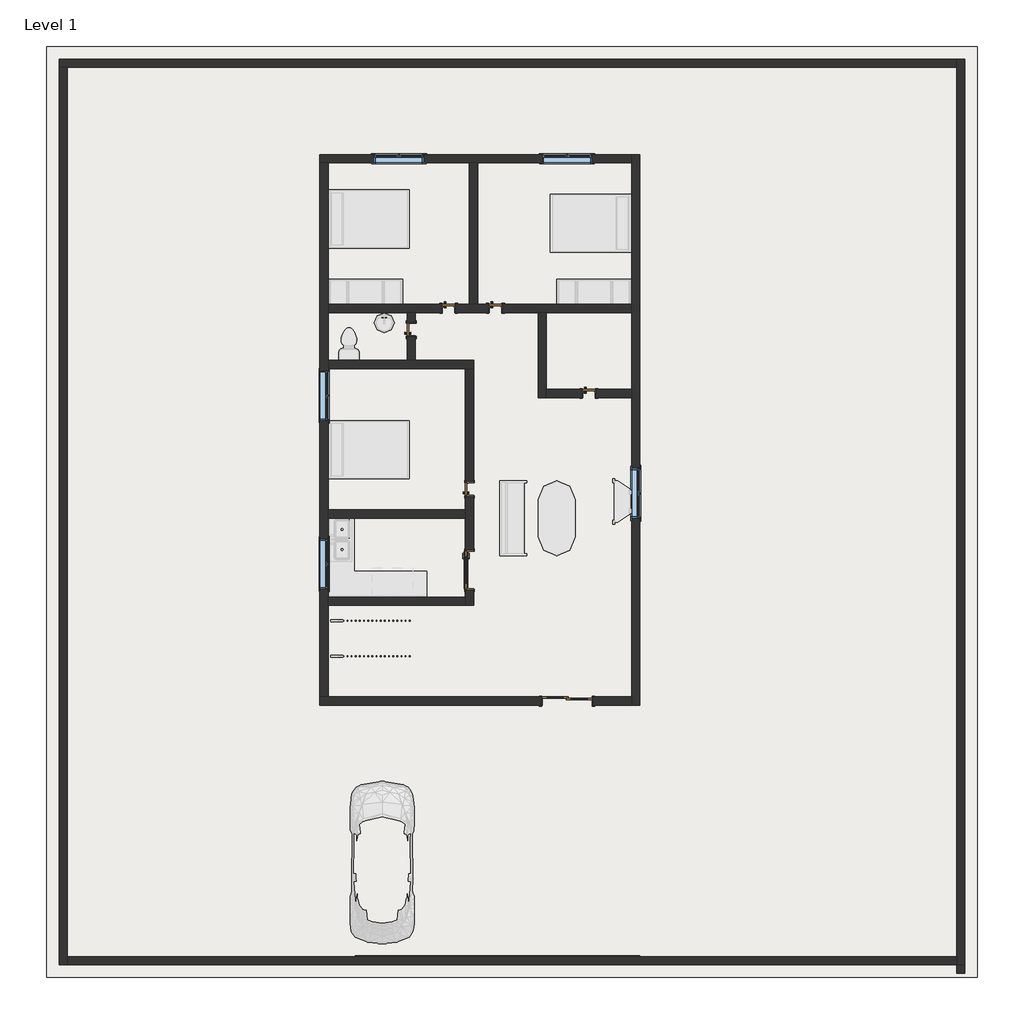
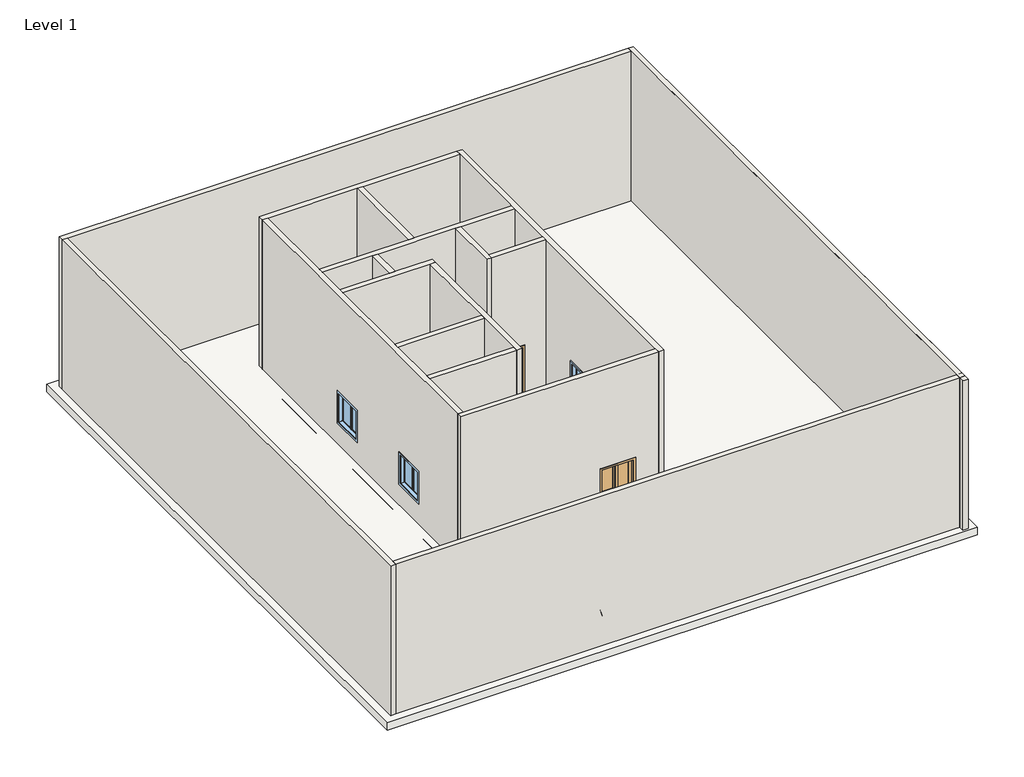
# One storey, part 1 of 3: 21 walls, 7 doors, 5 windows, 2 slabs.
"""IFC4 building model written with IfcOpenShell, lengths in millimetres."""

from ifc_helpers import new_model, si_unit, frame, origin, origin_with_axes, place, context, project, spatial, polyline, outline, extrude, faceted_brep, transform, mapped, element, save
from components import door_1768e003, door_f9cb40a9, door_5a382651, window_0862ab64

model = new_model("IFC4")

# Units and contexts
model_context = context("Model", 3, world=origin())
ifc_project = project(units=[si_unit("LENGTHUNIT", "METRE", prefix="MILLI")], contexts=[model_context])

# Site, building, storey
site = spatial("IfcSite", under=ifc_project)
building = spatial("IfcBuilding", under=site)
storey = spatial("IfcBuildingStorey", under=building, Name="Level 1", Elevation=0.0)

# Doors
placement = place(None, origin())
door_shape = door_1768e003(model_context)
element("IfcDoor", 1, ObjectType="36\" x 80\"", at=placement, inside=storey, context=model_context, shape_type="MappedRepresentation", body=[
    mapped(door_shape, transform((-7446.4010462, -2064.5818688, 0.0), x_axis=(0.0, 1.0, 0.0), y_axis=(-1.0, 0.0, 0.0), z_axis=(0.0, 0.0, 1.0))),
])
door_2_shape = door_f9cb40a9(model_context)
element("IfcDoor", 2, ObjectType="Door-Interior-Double-Sliding-2_Panel-Wood : 48\" x 80\"", at=placement, inside=storey, context=model_context, shape_type="MappedRepresentation", body=[
    mapped(door_2_shape, transform((-5055.6260462, -5261.8068688, 0.0), x_axis=(1.0, 0.0, 0.0), y_axis=(0.0, 1.0, 0.0), z_axis=(0.0, 0.0, 1.0))),
])
door_3_shape = door_5a382651(model_context)
element("IfcDoor", 3, ObjectType="Door-Interior-Single-5_Panel_Vert-Wood : 12\" x 80\"", at=placement, inside=storey, context=model_context, shape_type="MappedRepresentation", body=[
    mapped(door_3_shape, transform((-7951.2260462, 4339.3931312, 0.0), x_axis=(1.0, 0.0, 0.0), y_axis=(0.0, 1.0, 0.0), z_axis=(0.0, 0.0, 1.0))),
])
element("IfcDoor", 4, ObjectType="Door-Interior-Single-5_Panel_Vert-Wood : 12\" x 80\"", at=placement, inside=storey, context=model_context, shape_type="MappedRepresentation", body=[
    mapped(door_3_shape, transform((-6808.2260462, 4339.3931312, 0.0), x_axis=(1.0, 0.0, 0.0), y_axis=(0.0, 1.0, 0.0), z_axis=(0.0, 0.0, 1.0))),
])
element("IfcDoor", 5, ObjectType="Door-Interior-Single-5_Panel_Vert-Wood : 12\" x 80\"", at=placement, inside=storey, context=model_context, shape_type="MappedRepresentation", body=[
    mapped(door_3_shape, transform((-8868.8010462, 3815.5181312, 0.0), x_axis=(0.0, 1.0, 0.0), y_axis=(-1.0, 0.0, 0.0), z_axis=(0.0, 0.0, 1.0))),
])
element("IfcDoor", 6, ObjectType="Door-Interior-Single-5_Panel_Vert-Wood : 12\" x 80\"", at=placement, inside=storey, context=model_context, shape_type="MappedRepresentation", body=[
    mapped(door_3_shape, transform((-4522.2260462, 2256.5931312, 0.0), x_axis=(1.0, 0.0, 0.0), y_axis=(0.0, 1.0, 0.0), z_axis=(0.0, 0.0, 1.0))),
])
element("IfcDoor", 7, ObjectType="Door-Interior-Single-5_Panel_Vert-Wood : 12\" x 80\"", at=placement, inside=storey, context=model_context, shape_type="MappedRepresentation", body=[
    mapped(door_3_shape, transform((-7446.4010462, -83.3818688, 0.0), x_axis=(0.0, 1.0, 0.0), y_axis=(-1.0, 0.0, 0.0), z_axis=(0.0, 0.0, 1.0))),
])

# Slabs
element("IfcSlab", 8, ObjectType="Generic - 12\"", at=placement, inside=storey, context=model_context, shape_type="SweptSolid", body=[
    extrude(outline(polyline([(-11405.6260462, 8400.2181312), (-2972.8260462, 8400.2181312), (-2972.8260462, -5671.3818688), (-11405.6260462, -5671.3818688), (-11405.6260462, 8400.2181312)])), frame((0.0, 0.0, -304.8), z_axis=(0.0, 0.0, 1.0), x_axis=(1.0, 0.0, 0.0)), (0.0, 0.0, 1.0), 304.8),
])
element("IfcSlab", 9, ObjectType="Generic - 12\"", at=placement, inside=storey, context=model_context, shape_type="SweptSolid", body=[
    extrude(outline(polyline([(-17782.399436, -12021.3818688), (-17782.399436, 10737.0181312), (4976.000564, 10737.0181312), (4976.000564, -12021.3818688), (-17782.399436, -12021.3818688)])), frame((0.0, 0.0, -304.8), z_axis=(0.0, 0.0, 1.0), x_axis=(1.0, 0.0, 0.0)), (0.0, 0.0, 1.0), 304.8),
])

# Walls
element("IfcWall", 10, ObjectType="Generic - 8\"", at=placement, inside=storey, context=model_context, shape_type="Brep", body=[
    faceted_brep([(-11100.8260462, 7892.2181312, 0.0), (-10897.6260462, 7892.2181312, 0.0), (-7443.2260462, 7892.2181312, 0.0), (-7240.0260462, 7892.2181312, 0.0), (-3480.8260462, 7892.2181312, 0.0), (-3480.8260462, 7892.2181312, 6096.0), (-7240.0260462, 7892.2181312, 6096.0), (-7443.2260462, 7892.2181312, 6096.0), (-10897.6260462, 7892.2181312, 6096.0), (-11100.8260462, 7892.2181312, 6096.0), (-8560.8260462, 7892.2181312, 2133.6), (-8560.8260462, 7892.2181312, 914.4), (-9780.0260462, 7892.2181312, 914.4), (-9780.0260462, 7892.2181312, 2133.6), (-4446.0260462, 7892.2181312, 2133.6), (-4446.0260462, 7892.2181312, 914.4), (-5665.2260462, 7892.2181312, 914.4), (-5665.2260462, 7892.2181312, 2133.6), (-11100.8260462, 8095.4181312, 0.0), (-11100.8260462, 8095.4181312, 6096.0), (-3480.8260462, 8095.4181312, 6096.0), (-3480.8260462, 8095.4181312, 0.0), (-8560.8260462, 8095.4181312, 2133.6), (-9780.0260462, 8095.4181312, 2133.6), (-9780.0260462, 8095.4181312, 914.4), (-8560.8260462, 8095.4181312, 914.4), (-4446.0260462, 8095.4181312, 2133.6), (-5665.2260462, 8095.4181312, 2133.6), (-5665.2260462, 8095.4181312, 914.4), (-4446.0260462, 8095.4181312, 914.4)], [[[0, 1, 2, 3, 4, 5, 6, 7, 8, 9], [10, 11, 12, 13], [14, 15, 16, 17]], [[18, 19, 20, 21], [22, 23, 24, 25], [26, 27, 28, 29]], [[4, 3, 2, 1, 0, 18, 21]], [[9, 8, 7, 6, 5, 20, 19]], [[0, 9, 19, 18]], [[5, 4, 21, 20]], [[11, 10, 22, 25]], [[12, 11, 25, 24]], [[13, 12, 24, 23]], [[10, 13, 23, 22]], [[15, 14, 26, 29]], [[16, 15, 29, 28]], [[17, 16, 28, 27]], [[14, 17, 27, 26]]]),
])
element("IfcWall", 11, ObjectType="Generic - 8\"", at=placement, inside=storey, context=model_context, shape_type="Brep", body=[
    faceted_brep([(-3480.8260462, 8095.4181312, 0.0), (-3480.8260462, 7892.2181312, 0.0), (-3480.8260462, 4437.8181312, 0.0), (-3480.8260462, 4234.6181312, 0.0), (-3480.8260462, 2355.0181312, 0.0), (-3480.8260462, 2151.8181312, 0.0), (-3480.8260462, -5163.3818688, 0.0), (-3480.8260462, -5366.5818688, 0.0), (-3480.8260462, -5366.5818688, 6096.0), (-3480.8260462, -5163.3818688, 6096.0), (-3480.8260462, 2151.8181312, 6096.0), (-3480.8260462, 2355.0181312, 6096.0), (-3480.8260462, 4234.6181312, 6096.0), (-3480.8260462, 4437.8181312, 6096.0), (-3480.8260462, 7892.2181312, 6096.0), (-3480.8260462, 8095.4181312, 6096.0), (-3480.8260462, -794.5818688, 2133.6), (-3480.8260462, -794.5818688, 914.4), (-3480.8260462, 424.6181312, 914.4), (-3480.8260462, 424.6181312, 2133.6), (-3277.6260462, 8095.4181312, 0.0), (-3277.6260462, 8095.4181312, 6096.0), (-3277.6260462, -5366.5818688, 6096.0), (-3277.6260462, -5366.5818688, 0.0), (-3277.6260462, -794.5818688, 2133.6), (-3277.6260462, 424.6181312, 2133.6), (-3277.6260462, 424.6181312, 914.4), (-3277.6260462, -794.5818688, 914.4)], [[[0, 1, 2, 3, 4, 5, 6, 7, 8, 9, 10, 11, 12, 13, 14, 15], [16, 17, 18, 19]], [[20, 21, 22, 23], [24, 25, 26, 27]], [[7, 6, 5, 4, 3, 2, 1, 0, 20, 23]], [[15, 14, 13, 12, 11, 10, 9, 8, 22, 21]], [[8, 7, 23, 22]], [[0, 15, 21, 20]], [[17, 16, 24, 27]], [[18, 17, 27, 26]], [[19, 18, 26, 25]], [[16, 19, 25, 24]]]),
])
element("IfcWall", 12, ObjectType="Generic - 8\"", at=placement, inside=storey, context=model_context, shape_type="Brep", body=[
    faceted_brep([(-11100.8260462, -5163.3818688, 6096.0), (-10897.6260462, -5163.3818688, 6096.0), (-3480.8260462, -5163.3818688, 6096.0), (-3480.8260462, -5163.3818688, 0.0), (-4420.6260462, -5163.3818688, 0.0), (-4420.6260462, -5163.3818688, 2057.4), (-5690.6260462, -5163.3818688, 2057.4), (-5690.6260462, -5163.3818688, 0.0), (-10897.6260462, -5163.3818688, 0.0), (-11100.8260462, -5163.3818688, 0.0), (-3480.8260462, -5366.5818688, 6096.0), (-11100.8260462, -5366.5818688, 6096.0), (-11100.8260462, -5366.5818688, 0.0), (-5690.6260462, -5366.5818688, 0.0), (-5690.6260462, -5366.5818688, 2057.4), (-4420.6260462, -5366.5818688, 2057.4), (-4420.6260462, -5366.5818688, 0.0), (-3480.8260462, -5366.5818688, 0.0)], [[[0, 1, 2, 3, 4, 5, 6, 7, 8, 9]], [[10, 11, 12, 13, 14, 15, 16, 17]], [[3, 17, 16, 4]], [[12, 9, 8, 7, 13]], [[2, 1, 0, 11, 10]], [[3, 2, 10, 17]], [[0, 9, 12, 11]], [[15, 5, 4, 16]], [[5, 15, 14, 6]], [[6, 14, 13, 7]]]),
])
element("IfcWall", 13, ObjectType="Generic - 8\"", at=placement, inside=storey, context=model_context, shape_type="Brep", body=[
    faceted_brep([(-10897.6260462, -5163.3818688, 0.0), (-10897.6260462, -2928.1818688, 0.0), (-10897.6260462, -2724.9818688, 0.0), (-10897.6260462, -794.5818688, 0.0), (-10897.6260462, -591.3818688, 0.0), (-10897.6260462, 2863.0181312, 0.0), (-10897.6260462, 3066.2181312, 0.0), (-10897.6260462, 4234.6181312, 0.0), (-10897.6260462, 4437.8181312, 0.0), (-10897.6260462, 7892.2181312, 0.0), (-10897.6260462, 7892.2181312, 6096.0), (-10897.6260462, 4437.8181312, 6096.0), (-10897.6260462, 4234.6181312, 6096.0), (-10897.6260462, 3066.2181312, 6096.0), (-10897.6260462, 2863.0181312, 6096.0), (-10897.6260462, -591.3818688, 6096.0), (-10897.6260462, -794.5818688, 6096.0), (-10897.6260462, -2724.9818688, 6096.0), (-10897.6260462, -2928.1818688, 6096.0), (-10897.6260462, -5163.3818688, 6096.0), (-10897.6260462, -2521.7818688, 2133.6), (-10897.6260462, -1302.5818688, 2133.6), (-10897.6260462, -1302.5818688, 914.4), (-10897.6260462, -2521.7818688, 914.4), (-10897.6260462, 1593.0181312, 2133.6), (-10897.6260462, 2812.2181312, 2133.6), (-10897.6260462, 2812.2181312, 914.4), (-10897.6260462, 1593.0181312, 914.4), (-11100.8260462, -5163.3818688, 0.0), (-11100.8260462, -5163.3818688, 6096.0), (-11100.8260462, 7892.2181312, 6096.0), (-11100.8260462, 7892.2181312, 0.0), (-11100.8260462, -2521.7818688, 2133.6), (-11100.8260462, -2521.7818688, 914.4), (-11100.8260462, -1302.5818688, 914.4), (-11100.8260462, -1302.5818688, 2133.6), (-11100.8260462, 1593.0181312, 2133.6), (-11100.8260462, 1593.0181312, 914.4), (-11100.8260462, 2812.2181312, 914.4), (-11100.8260462, 2812.2181312, 2133.6)], [[[0, 1, 2, 3, 4, 5, 6, 7, 8, 9, 10, 11, 12, 13, 14, 15, 16, 17, 18, 19], [20, 21, 22, 23], [24, 25, 26, 27]], [[28, 29, 30, 31], [32, 33, 34, 35], [36, 37, 38, 39]], [[9, 8, 7, 6, 5, 4, 3, 2, 1, 0, 28, 31]], [[19, 18, 17, 16, 15, 14, 13, 12, 11, 10, 30, 29]], [[10, 9, 31, 30]], [[0, 19, 29, 28]], [[33, 32, 20, 23]], [[34, 33, 23, 22]], [[35, 34, 22, 21]], [[32, 35, 21, 20]], [[37, 36, 24, 27]], [[38, 37, 27, 26]], [[39, 38, 26, 25]], [[36, 39, 25, 24]]]),
])
element("IfcWall", 14, ObjectType="Generic - 8\"", at=placement, inside=storey, context=model_context, shape_type="Brep", body=[
    faceted_brep([(-3480.8260462, 4234.6181312, 6096.0), (-5563.6260462, 4234.6181312, 6096.0), (-5766.8260462, 4234.6181312, 6096.0), (-8764.0260462, 4234.6181312, 6096.0), (-8967.2260462, 4234.6181312, 6096.0), (-10897.6260462, 4234.6181312, 6096.0), (-10897.6260462, 4234.6181312, 0.0), (-8967.2260462, 4234.6181312, 0.0), (-8764.0260462, 4234.6181312, 0.0), (-8129.0260462, 4234.6181312, 0.0), (-8129.0260462, 4234.6181312, 2057.4), (-7773.4260462, 4234.6181312, 2057.4), (-7773.4260462, 4234.6181312, 0.0), (-6986.0260462, 4234.6181312, 0.0), (-6986.0260462, 4234.6181312, 2057.4), (-6630.4260462, 4234.6181312, 2057.4), (-6630.4260462, 4234.6181312, 0.0), (-5766.8260462, 4234.6181312, 0.0), (-5563.6260462, 4234.6181312, 0.0), (-3480.8260462, 4234.6181312, 0.0), (-10897.6260462, 4437.8181312, 6096.0), (-7443.2260462, 4437.8181312, 6096.0), (-7240.0260462, 4437.8181312, 6096.0), (-3480.8260462, 4437.8181312, 6096.0), (-3480.8260462, 4437.8181312, 0.0), (-6630.4260462, 4437.8181312, 0.0), (-6630.4260462, 4437.8181312, 2057.4), (-6986.0260462, 4437.8181312, 2057.4), (-6986.0260462, 4437.8181312, 0.0), (-7240.0260462, 4437.8181312, 0.0), (-7443.2260462, 4437.8181312, 0.0), (-7773.4260462, 4437.8181312, 0.0), (-7773.4260462, 4437.8181312, 2057.4), (-8129.0260462, 4437.8181312, 2057.4), (-8129.0260462, 4437.8181312, 0.0), (-10897.6260462, 4437.8181312, 0.0)], [[[0, 1, 2, 3, 4, 5, 6, 7, 8, 9, 10, 11, 12, 13, 14, 15, 16, 17, 18, 19]], [[20, 21, 22, 23, 24, 25, 26, 27, 28, 29, 30, 31, 32, 33, 34, 35]], [[6, 35, 34, 9, 8, 7]], [[24, 19, 18, 17, 16, 25]], [[12, 31, 30, 29, 28, 13]], [[5, 4, 3, 2, 1, 0, 23, 22, 21, 20]], [[0, 19, 24, 23]], [[6, 5, 20, 35]], [[11, 32, 31, 12]], [[32, 11, 10, 33]], [[33, 10, 9, 34]], [[15, 26, 25, 16]], [[26, 15, 14, 27]], [[27, 14, 13, 28]]]),
])
element("IfcWall", 15, ObjectType="Generic - 8\"", at=placement, inside=storey, context=model_context, shape_type="SweptSolid", body=[
    extrude(outline(polyline([(-7443.2260462, 7892.2181312), (-7240.0260462, 7892.2181312), (-7240.0260462, 4437.8181312), (-7443.2260462, 4437.8181312), (-7443.2260462, 7892.2181312)])), origin_with_axes(), (0.0, 0.0, 1.0), 6096.0),
])
element("IfcWall", 16, ObjectType="Generic - 8\"", at=placement, inside=storey, context=model_context, shape_type="Brep", body=[
    faceted_brep([(-10897.6260462, 2863.0181312, 0.0), (-7544.8260462, 2863.0181312, 0.0), (-7341.6260462, 2863.0181312, 0.0), (-7341.6260462, 2863.0181312, 6096.0), (-7544.8260462, 2863.0181312, 6096.0), (-10897.6260462, 2863.0181312, 6096.0), (-10897.6260462, 3066.2181312, 0.0), (-10897.6260462, 3066.2181312, 6096.0), (-8967.2260462, 3066.2181312, 6096.0), (-8764.0260462, 3066.2181312, 6096.0), (-7341.6260462, 3066.2181312, 6096.0), (-7341.6260462, 3066.2181312, 0.0), (-8764.0260462, 3066.2181312, 0.0), (-8967.2260462, 3066.2181312, 0.0)], [[[0, 1, 2, 3, 4, 5]], [[6, 7, 8, 9, 10, 11, 12, 13]], [[2, 1, 0, 6, 13, 12, 11]], [[3, 2, 11, 10]], [[5, 4, 3, 10, 9, 8, 7]], [[0, 5, 7, 6]]]),
])
element("IfcWall", 17, ObjectType="Generic - 8\"", at=placement, inside=storey, context=model_context, shape_type="SweptSolid", body=[
    extrude(outline(polyline([(4234.6181312, 6096.0), (4234.6181312, 0.0), (3993.3181312, 0.0), (3993.3181312, 2057.4), (3637.7181312, 2057.4), (3637.7181312, 0.0), (3066.2181312, 0.0), (3066.2181312, 6096.0), (4234.6181312, 6096.0)])), frame((-8967.2260462, 0.0, 0.0), z_axis=(1.0, 0.0, 0.0), x_axis=(0.0, 1.0, 0.0)), (0.0, 0.0, 1.0), 203.2),
])
element("IfcWall", 18, ObjectType="Generic - 8\"", at=placement, inside=storey, context=model_context, shape_type="SweptSolid", body=[
    extrude(outline(polyline([(-7443.2260462, 7892.2181312), (-7240.0260462, 7892.2181312), (-7240.0260462, 4437.8181312), (-7443.2260462, 4437.8181312), (-7443.2260462, 7892.2181312)])), origin_with_axes(), (0.0, 0.0, 1.0), 6096.0),
])
element("IfcWall", 19, ObjectType="Generic - 8\"", at=placement, inside=storey, context=model_context, shape_type="Brep", body=[
    faceted_brep([(-7544.8260462, -2928.1818688, 6096.0), (-7544.8260462, -2724.9818688, 6096.0), (-7544.8260462, -794.5818688, 6096.0), (-7544.8260462, -591.3818688, 6096.0), (-7544.8260462, 2863.0181312, 6096.0), (-7544.8260462, 2863.0181312, 0.0), (-7544.8260462, 94.4181312, 0.0), (-7544.8260462, 94.4181312, 2057.4), (-7544.8260462, -261.1818688, 2057.4), (-7544.8260462, -261.1818688, 0.0), (-7544.8260462, -591.3818688, 0.0), (-7544.8260462, -794.5818688, 0.0), (-7544.8260462, -1581.9818688, 0.0), (-7544.8260462, -1581.9818688, 2057.4), (-7544.8260462, -2547.1818688, 2057.4), (-7544.8260462, -2547.1818688, 0.0), (-7544.8260462, -2724.9818688, 0.0), (-7544.8260462, -2928.1818688, 0.0), (-7341.6260462, 2863.0181312, 6096.0), (-7341.6260462, -2928.1818688, 6096.0), (-7341.6260462, -2928.1818688, 0.0), (-7341.6260462, -2547.1818688, 0.0), (-7341.6260462, -2547.1818688, 2057.4), (-7341.6260462, -1581.9818688, 2057.4), (-7341.6260462, -1581.9818688, 0.0), (-7341.6260462, -261.1818688, 0.0), (-7341.6260462, -261.1818688, 2057.4), (-7341.6260462, 94.4181312, 2057.4), (-7341.6260462, 94.4181312, 0.0), (-7341.6260462, 2863.0181312, 0.0)], [[[0, 1, 2, 3, 4, 5, 6, 7, 8, 9, 10, 11, 12, 13, 14, 15, 16, 17]], [[18, 19, 20, 21, 22, 23, 24, 25, 26, 27, 28, 29]], [[5, 29, 28, 6]], [[20, 17, 16, 15, 21]], [[24, 12, 11, 10, 9, 25]], [[4, 3, 2, 1, 0, 19, 18]], [[5, 4, 18, 29]], [[0, 17, 20, 19]], [[23, 13, 12, 24]], [[13, 23, 22, 14]], [[14, 22, 21, 15]], [[27, 7, 6, 28]], [[7, 27, 26, 8]], [[8, 26, 25, 9]]]),
])
element("IfcWall", 20, ObjectType="Generic - 8\"", at=placement, inside=storey, context=model_context, shape_type="SweptSolid", body=[
    extrude(outline(polyline([(-10897.6260462, -591.3818688), (-7544.8260462, -591.3818688), (-7544.8260462, -794.5818688), (-10897.6260462, -794.5818688), (-10897.6260462, -591.3818688)])), origin_with_axes(), (0.0, 0.0, 1.0), 6096.0),
])
element("IfcWall", 21, ObjectType="Generic - 8\"", at=placement, inside=storey, context=model_context, shape_type="SweptSolid", body=[
    extrude(outline(polyline([(-10897.6260462, -2724.9818688), (-7544.8260462, -2724.9818688), (-7544.8260462, -2928.1818688), (-10897.6260462, -2928.1818688), (-10897.6260462, -2724.9818688)])), origin_with_axes(), (0.0, 0.0, 1.0), 6096.0),
])
element("IfcWall", 22, ObjectType="Generic - 8\"", at=placement, inside=storey, context=model_context, shape_type="Brep", body=[
    faceted_brep([(-5766.8260462, 4234.6181312, 0.0), (-5766.8260462, 2151.8181312, 0.0), (-5766.8260462, 2151.8181312, 6096.0), (-5766.8260462, 4234.6181312, 6096.0), (-5563.6260462, 4234.6181312, 0.0), (-5563.6260462, 4234.6181312, 6096.0), (-5563.6260462, 2355.0181312, 6096.0), (-5563.6260462, 2151.8181312, 6096.0), (-5563.6260462, 2151.8181312, 0.0), (-5563.6260462, 2355.0181312, 0.0)], [[[0, 1, 2, 3]], [[4, 5, 6, 7, 8, 9]], [[1, 0, 4, 9, 8]], [[3, 2, 7, 6, 5]], [[0, 3, 5, 4]], [[2, 1, 8, 7]]]),
])
element("IfcWall", 23, ObjectType="Generic - 8\"", at=placement, inside=storey, context=model_context, shape_type="SweptSolid", body=[
    extrude(outline(polyline([(6096.0, -3480.8260462), (6096.0, -5563.6260462), (0.0, -5563.6260462), (0.0, -4700.0260462), (2057.4, -4700.0260462), (2057.4, -4344.4260462), (0.0, -4344.4260462), (0.0, -3480.8260462), (6096.0, -3480.8260462)])), frame((0.0, 2151.8181312, 0.0), z_axis=(0.0, 1.0, 0.0), x_axis=(0.0, 0.0, 1.0)), (0.0, 0.0, 1.0), 203.2),
])
element("IfcWall", 24, ObjectType="Generic - 8\"", at=placement, inside=storey, context=model_context, shape_type="Brep", body=[
    faceted_brep([(4671.200564, -11716.5818688, 0.0), (4671.200564, 10432.2181312, 0.0), (4671.200564, 10432.2181312, 6096.0), (4671.200564, -11716.5818688, 6096.0), (4468.000564, -11716.5818688, 0.0), (4468.000564, -11716.5818688, 6096.0), (4468.000564, -11513.3818688, 6096.0), (4468.000564, 10229.0181312, 6096.0), (4468.000564, 10432.2181312, 6096.0), (4468.000564, 10432.2181312, 0.0), (4468.000564, 10229.0181312, 0.0), (4468.000564, -11513.3818688, 0.0)], [[[0, 1, 2, 3]], [[4, 5, 6, 7, 8, 9, 10, 11]], [[1, 0, 4, 11, 10, 9]], [[3, 2, 8, 7, 6, 5]], [[2, 1, 9, 8]], [[0, 3, 5, 4]]]),
])
element("IfcWall", 25, ObjectType="Generic - 8\"", at=placement, inside=storey, context=model_context, shape_type="Brep", body=[
    faceted_brep([(4468.000564, 10432.2181312, 0.0), (-17477.599436, 10432.2181312, 0.0), (-17477.599436, 10432.2181312, 6096.0), (4468.000564, 10432.2181312, 6096.0), (4468.000564, 10229.0181312, 0.0), (4468.000564, 10229.0181312, 6096.0), (-17274.399436, 10229.0181312, 6096.0), (-17477.599436, 10229.0181312, 6096.0), (-17477.599436, 10229.0181312, 0.0), (-17274.399436, 10229.0181312, 0.0)], [[[0, 1, 2, 3]], [[4, 5, 6, 7, 8, 9]], [[1, 0, 4, 9, 8]], [[3, 2, 7, 6, 5]], [[0, 3, 5, 4]], [[2, 1, 8, 7]]]),
])
element("IfcWall", 26, ObjectType="Generic - 8\"", at=placement, inside=storey, context=model_context, shape_type="Brep", body=[
    faceted_brep([(-17477.599436, 10229.0181312, 0.0), (-17477.599436, -11716.5818688, 0.0), (-17477.599436, -11716.5818688, 6096.0), (-17477.599436, 10229.0181312, 6096.0), (-17274.399436, 10229.0181312, 0.0), (-17274.399436, 10229.0181312, 6096.0), (-17274.399436, -11513.3818688, 6096.0), (-17274.399436, -11716.5818688, 6096.0), (-17274.399436, -11716.5818688, 0.0), (-17274.399436, -11513.3818688, 0.0)], [[[0, 1, 2, 3]], [[4, 5, 6, 7, 8, 9]], [[1, 0, 4, 9, 8]], [[3, 2, 7, 6, 5]], [[0, 3, 5, 4]], [[2, 1, 8, 7]]]),
])
element("IfcWall", 27, ObjectType="Generic - 8\"", at=placement, inside=storey, context=model_context, shape_type="SweptSolid", body=[
    extrude(outline(polyline([(4468.000564, -11716.5818688), (-17274.399436, -11716.5818688), (-17274.399436, -11513.3818688), (4468.000564, -11513.3818688), (4468.000564, -11716.5818688)])), origin_with_axes(), (0.0, 0.0, 1.0), 6096.0),
])
element("IfcWall", 28, ObjectType="Generic - 8\"", at=placement, inside=storey, context=model_context, shape_type="SweptSolid", body=[
    extrude(outline(polyline([(4671.200564, 10229.0181312), (4671.200564, -11513.3818688), (4468.000564, -11513.3818688), (4468.000564, 10229.0181312), (4671.200564, 10229.0181312)])), origin_with_axes(), (0.0, 0.0, 1.0), 6096.0),
])
element("IfcWall", 29, ObjectType="Generic - 8\"", at=placement, inside=storey, context=model_context, shape_type="SweptSolid", body=[
    extrude(outline(polyline([(4671.200564, 10025.8181312), (4671.200564, -11919.7818688), (4468.000564, -11919.7818688), (4468.000564, 10025.8181312), (4671.200564, 10025.8181312)])), origin_with_axes(), (0.0, 0.0, 1.0), 6096.0),
])
element("IfcWall", 30, ObjectType="Generic - 8\"", at=placement, inside=storey, context=model_context, shape_type="SweptSolid", body=[
    extrude(outline(polyline([(-17274.399436, 10432.2181312), (4468.000564, 10432.2181312), (4468.000564, 10229.0181312), (-17274.399436, 10229.0181312), (-17274.399436, 10432.2181312)])), origin_with_axes(), (0.0, 0.0, 1.0), 6096.0),
])

# Windows
window_shape = window_0862ab64(model_context)
element("IfcWindow", 31, ObjectType="Casement Dbl with Trim : 48\" x 48\"", at=placement, inside=storey, context=model_context, shape_type="MappedRepresentation", body=[
    mapped(window_shape, transform((-11018.2760462, -1912.1818688, 0.0), x_axis=(0.0, -1.0, 0.0), y_axis=(1.0, 0.0, 0.0), z_axis=(0.0, 0.0, 1.0))),
])
element("IfcWindow", 32, ObjectType="Casement Dbl with Trim : 48\" x 48\"", at=placement, inside=storey, context=model_context, shape_type="MappedRepresentation", body=[
    mapped(window_shape, transform((-11018.2760462, 2202.6181312, 0.0), x_axis=(0.0, -1.0, 0.0), y_axis=(1.0, 0.0, 0.0), z_axis=(0.0, 0.0, 1.0))),
])
element("IfcWindow", 33, ObjectType="Casement Dbl with Trim : 48\" x 48\"", at=placement, inside=storey, context=model_context, shape_type="MappedRepresentation", body=[
    mapped(window_shape, transform((-9170.4260462, 7974.7681312, 0.0), x_axis=(1.0, 0.0, 0.0), y_axis=(0.0, 1.0, 0.0), z_axis=(0.0, 0.0, 1.0))),
])
element("IfcWindow", 34, ObjectType="Casement Dbl with Trim : 48\" x 48\"", at=placement, inside=storey, context=model_context, shape_type="MappedRepresentation", body=[
    mapped(window_shape, transform((-5055.6260462, 7974.7681312, 0.0), x_axis=(1.0, 0.0, 0.0), y_axis=(0.0, 1.0, 0.0), z_axis=(0.0, 0.0, 1.0))),
])
element("IfcWindow", 35, ObjectType="Casement Dbl with Trim : 48\" x 48\"", at=placement, inside=storey, context=model_context, shape_type="MappedRepresentation", body=[
    mapped(window_shape, transform((-3398.2760462, -184.9818688, 0.0), x_axis=(0.0, -1.0, 0.0), y_axis=(1.0, 0.0, 0.0), z_axis=(0.0, 0.0, 1.0))),
])

save(model, "model.ifc")

# Revit data of these elements
# Type "36\" x 80\""
#   Type Mark = "8"
#   Assembly Code = "B2030100"
#   Analytic Construction = "French door, wood frame with single glass"
#   Threshold Offset [instance default] = 0' - 0 1/2"
#   Thickness = 0' - 1 3/8"
#   Thermal Resistance (R) = 1.0696 (h·ft²·°F)/BTU
#   Swing Angle [instance default] = 90.00°
#   Stiles = 0' - 4 3/4"
#   Rough Width = 3' - 2"
#   Rough Height = 6' - 9"
#   Radius = 1' - 8.05625"
#   Lock Rail = 0' - 7 1/8"
#   Height = 6' - 8"
#   Width = 3' - 0"
#   Heat Transfer Coefficient (U) = 0.9350 BTU/(h·ft²·°F)
#   Door Offset [instance default] = 0' - 0"
#   Bottom Rail = 0' - 9 1/2"
#   Threshold [instance default] = yes
#   Function = 1
#   Exterior Trim [instance default] = yes
#   Trim Material = Cherry
#   Threshold Material = Cherry
#   Panel Material = Cherry
#   Glazing = Glass
#   Frame Material = Cherry
#   Door Handle Material = Aluminum
#   Visual Light Transmittance = 0
#   Solar Heat Gain Coefficient = 0
#   Wall Closure = (empty or 0)
#   Construction Type = (empty or 0)
# Type "Door-Interior-Double-Sliding-2_Panel-Wood : 48\" x 80\""
#   Type Mark = "10"
#   Assembly Code = "C1020300"
#   Analytic Construction = "Wooden"
#   Top Rail = 0' - 4 11/16"
#   Thickness = 0' - 1 3/8"
#   Thermal Resistance (R) = 2.5876 (h·ft²·°F)/BTU
#   Stiles = 0' - 4 3/4"
#   Rough Width = 4' - 2"
#   Rough Height = 6' - 9"
#   Lock Rail = 0' - 7 1/2"
#   Height = 6' - 8"
#   Width = 4' - 0"
#   Heat Transfer Coefficient (U) = 0.3865 BTU/(h·ft²·°F)
#   Bottom Rail = 0' - 9 1/8"
#   Trim Material = Cherry
#   Panel Material = Cherry
#   Frame Material = Cherry
#   Visual Light Transmittance = 0
#   Solar Heat Gain Coefficient = 0
#   Wall Closure = (empty or 0)
#   Function = (empty or 0)
# Type "Door-Interior-Single-5_Panel_Vert-Wood : 12\" x 80\""
#   Type Mark = "9"
#   Assembly Code = "C1020300"
#   Analytic Construction = "Wooden"
#   Top Rail = 0' - 4 11/16"
#   Thickness = 0' - 1 3/8"
#   Thermal Resistance (R) = 2.5876 (h·ft²·°F)/BTU
#   Swing Angle [instance default] = 90.00°
#   Stiles = 0' - 2 3/8"
#   Rough Width = 1' - 2"
#   Rough Height = 6' - 9"
#   Intermediate Rail = 0' - 4 1/2"
#   Height = 6' - 8"
#   Width = 1' - 0"
#   Heat Transfer Coefficient (U) = 0.3865 BTU/(h·ft²·°F)
#   Bottom Rail = 0' - 9 1/8"
#   Trim Material = Cherry
#   Panel Material = Cherry
#   Frame Material = Cherry
#   Door Handle Material = Aluminum
#   Visual Light Transmittance = 0
#   Solar Heat Gain Coefficient = 0
#   Wall Closure = (empty or 0)
#   Function = (empty or 0)
# Type "Generic - 12\""
#   Assembly Code = "B1010"
#   Function = 0
#   Layers, outside or top first: 1' - 0" "Default New Material" (function 1)
# Type "Generic - 8\""
#   Assembly Code = "B2010"
#   Layers, outside or top first: 0' - 8" "Default New Material(1)" (function 1)
# Type "Casement Dbl with Trim : 48\" x 48\""
#   Type Mark = "10"
#   Construction Type Id = "GSP4R"
#   Assembly Code = "B2020100"
#   Analytic Construction = "1/8 in Pilkington single glazing"
#   Visual Light Transmittance = 0.9
#   Solar Heat Gain Coefficient = 0.78
#   Heat Transfer Coefficient (U) = 0.6496 BTU/(h·ft²·°F)
#   Height = 4' - 0"
#   Default Sill Height = 3' - 0"
#   Trim Projection - Ext. = 0' - 0 1/2"
#   Trim Projection - Int. = 0' - 0 3/4"
#   Trim Width - Exterior = 0' - 3 1/2"
#   Trim Width - Interior = 0' - 3 1/2"
#   Width = 4' - 0"
#   Window Inset = 0' - 0 3/4"
#   Define Thermal Properties by = 1
#   Glass Pane Material = Glass
#   Sash Material = Sash
#   Trim Exterior Material = Trim
#   Trim Interior Material = Trim
#   Wall Closure = (empty or 0)
# Element 1 (IfcDoor, "36\" x 80\"")
#   Threshold Offset = 0' - 0 1/2"
#   Swing Angle = 90.00°
#   Door Offset = 0' - 0"
#   Threshold = yes
#   Exterior Trim = yes
#   Phase Created = New Construction
#   Materials on its faces: "Cherry", "Aluminum", "Glass"
# Element 2 (IfcDoor, "Door-Interior-Double-Sliding-2_Panel-Wood : 48\" x 80\"")
#   Phase Created = New Construction
#   Materials on its faces: "Cherry"
# Elements 3, 4, 5, 6, 7 (IfcDoor, "Door-Interior-Single-5_Panel_Vert-Wood : 12\" x 80\"")
#   Swing Angle = 90.00°
#   Phase Created = New Construction
#   Materials on its faces: "Cherry", "Aluminum"
# Element 8 (IfcSlab, "Generic - 12\"")
#   built-in parameter 1001955 = 1.5708 (stored number, unit not read)
#   Height Offset From Level = 0' - 0"
#   Phase Created = New Construction
#   Materials on its faces: "Default New Material"
# Element 9 (IfcSlab, "Generic - 12\"")
#   built-in parameter 1001955 = -1.5708 (stored number, unit not read)
#   Height Offset From Level = 0' - 0"
#   Phase Created = New Construction
#   Materials on its faces: "Default New Material"
# Elements 10, 11, 12, 13, 14, 15, 16, 17, 18, 19, 20, 21, 22, 23, 24, 25, 26, 27, 28, 29, 30 (IfcWall, "Generic - 8\"")
#   Top Offset = 0' - 0"
#   Base Offset = 0' - 0"
#   Unconnected Height = 20' - 0"
#   wall height = 20' - 0"
#   Phase Created = New Construction
#   Base Constraint = Level 1
#   Materials on its faces: "Default New Material(1)"
# Element 31 (IfcWindow, "Casement Dbl with Trim : 48\" x 48\"")
#   Mark = "1"
#   Phase Created = New Construction
#   Materials on its faces: "Sash", "Trim", "Glass"
# Element 32 (IfcWindow, "Casement Dbl with Trim : 48\" x 48\"")
#   Mark = "2"
#   Phase Created = New Construction
#   Materials on its faces: "Sash", "Trim", "Glass"
# Element 33 (IfcWindow, "Casement Dbl with Trim : 48\" x 48\"")
#   Mark = "3"
#   Phase Created = New Construction
#   Materials on its faces: "Sash", "Trim", "Glass"
# Element 34 (IfcWindow, "Casement Dbl with Trim : 48\" x 48\"")
#   Mark = "4"
#   Phase Created = New Construction
#   Materials on its faces: "Sash", "Trim", "Glass"
# Element 35 (IfcWindow, "Casement Dbl with Trim : 48\" x 48\"")
#   Mark = "5"
#   Phase Created = New Construction
#   Materials on its faces: "Sash", "Trim", "Glass"
# Materials
#   "Cherry": class "Wood", colour RGB 226 177 128, transparency 0, Description = "Prunus Serotina", Cost = 0
#   "Glass": class "Glass", colour RGB 0 128 192, transparency 0.75, Description = "Soda Lime Glass", Cost = 0
#   "Aluminum": class "Metal", colour RGB 247 247 247, transparency 0, Description = "Aluminum 6061", Cost = 0
#   "Default New Material": class "Generic", colour RGB 120 120 120, transparency 0, Cost = 0
#   "Default New Material(1)": class "Generic", colour RGB 120 120 120, transparency 0, Cost = 0
#   "Sash": class "Wood", colour RGB 224 178 126, transparency 0
#   "Trim": class "Wood", colour RGB 224 178 126, transparency 0
